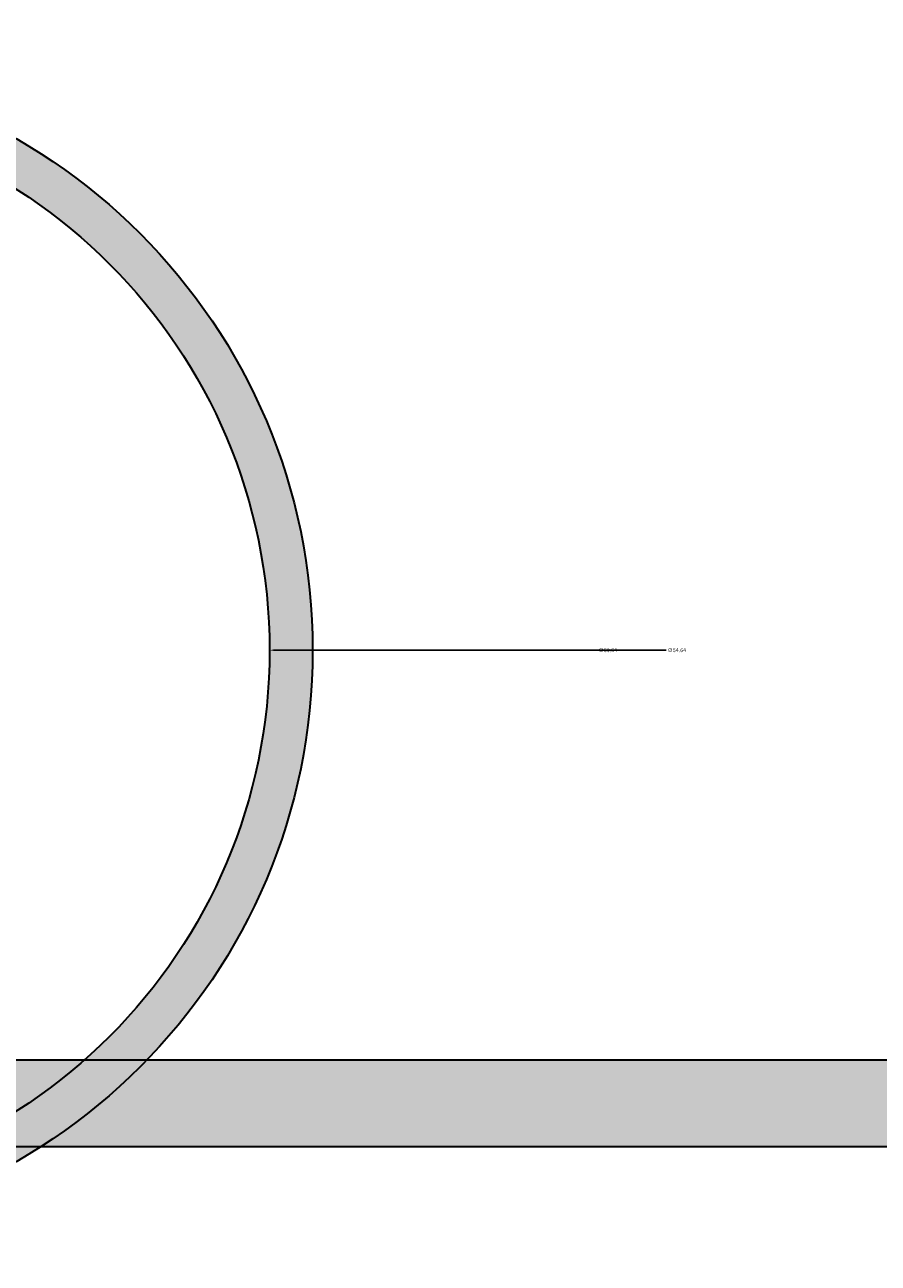
# Model space of a CAD drawing. Units: millimetres. Extents: x 446512 to 447461, y 70395 to 70610.
# Tile 31 of 39: x 447300 to 447340, y 70447 to 70505. Entities that reach past the tile are written whole.
import ezdxf

# ---------------------------------------------------------------- set-up
doc = ezdxf.new("R2010")
doc.units = ezdxf.units.MM
for name, color, linetype, lineweight in [('A-ANNO-DIMS', 2, 'Continuous', 18), ('A-FURN', 7, 'Continuous', 35), ('A-FURN-PATT', 38, 'Continuous', 13)]:
    doc.layers.add(name, color=color, linetype=linetype, lineweight=lineweight)
doc.styles.get("Standard").update_dxf_attribs({"font": 'arial.ttf'})
doc.dimstyles.get("Standard").update_dxf_attribs({"dimtxt": 0.18, "dimasz": 0.18, "dimexe": 0.18, "dimexo": 0.0625, "dimgap": 0.09, "dimtad": 0, "dimtih": 1, "dimtoh": 1, "dimdec": 4, "dimzin": 0, "dimdsep": 46, "dimtxsty": 'Standard', "dimcen": 0.09, "dimadec": 0, "dimazin": 0, "dimtfac": 1, "dimtdec": 4, "dimtofl": 0, "dimtmove": 0, "dimatfit": 3, "dimfxl": 1, "dimtolj": 1, "dimtzin": 0, "dimarcsym": 0})

# ---------------------------------------------------------------- blocks, each defined once
blk = doc.blocks.new('*D61')
at = {"layer": 'A-ANNO-DIMS', "color": 0, "lineweight": -2, "transparency": 16777216}
for p, q in [((447254.943, 70452.792), (447254.943, 70394.885)), ((447450.532, 70432.19), (447450.532, 70394.885)), ((447255.123, 70395.065), (447352.352, 70395.065)), ((447450.352, 70395.065), (447353.122, 70395.065))]:
    blk.add_line(p, q, dxfattribs=at)
at = {"layer": 'A-ANNO-DIMS', "color": 0, "transparency": 16777216}
for points in [[(447255.123, 70395.095), (447255.123, 70395.035), (447254.943, 70395.065)], [(447450.352, 70395.095), (447450.352, 70395.035), (447450.532, 70395.065)]]:
    blk.add_solid(points, dxfattribs=at)
at = {"layer": 'Defpoints', "color": 0, "transparency": 16777216}
for p in [(447254.943, 70452.855), (447450.532, 70432.253), (447450.532, 70395.065)]:
    blk.add_point(p, dxfattribs=at)
at = {"layer": 'A-ANNO-DIMS', "color": 0, "transparency": 16777216, "insert": (447352.737, 70395.065), "char_height": 0.18, "attachment_point": 5}
blk.add_mtext('\\A1;195.6', dxfattribs=at)
blk = doc.blocks.new('*D63')
at = {"layer": 'A-ANNO-DIMS', "color": 0, "lineweight": -2, "transparency": 16777216}
for p, q in [((447286.509, 70475.943), (447286.509, 70610.145)), ((447340.049, 70506.612), (447340.049, 70610.145)), ((447286.689, 70609.965), (447312.886, 70609.965)), ((447339.869, 70609.965), (447313.672, 70609.965))]:
    blk.add_line(p, q, dxfattribs=at)
at = {"layer": 'A-ANNO-DIMS', "color": 0, "transparency": 16777216}
for points in [[(447286.689, 70609.995), (447286.689, 70609.935), (447286.509, 70609.965)], [(447339.869, 70609.995), (447339.869, 70609.935), (447340.049, 70609.965)]]:
    blk.add_solid(points, dxfattribs=at)
at = {"layer": 'Defpoints', "color": 0, "transparency": 16777216}
for p in [(447340.049, 70609.965), (447340.049, 70506.55), (447286.509, 70475.881)]:
    blk.add_point(p, dxfattribs=at)
at = {"layer": 'A-ANNO-DIMS', "color": 0, "transparency": 16777216, "insert": (447313.279, 70609.965), "char_height": 0.18, "attachment_point": 5}
blk.add_mtext('\\A1;53.54', dxfattribs=at)
blk = doc.blocks.new('*D72')
at = {"layer": 'A-ANNO-DIMS', "color": 0, "lineweight": -2, "transparency": 16777216}
for p, q in [((447254.88, 70452.855), (447244.513, 70452.855)), ((447244.693, 70452.675), (447244.693, 70429.266)), ((447244.693, 70405.495), (447244.693, 70428.903)), ((447365.363, 70405.315), (447244.513, 70405.315))]:
    blk.add_line(p, q, dxfattribs=at)
at = {"layer": 'A-ANNO-DIMS', "color": 0, "transparency": 16777216}
for points in [[(447244.663, 70452.675), (447244.723, 70452.675), (447244.693, 70452.855)], [(447244.663, 70405.495), (447244.723, 70405.495), (447244.693, 70405.315)]]:
    blk.add_solid(points, dxfattribs=at)
at = {"layer": 'Defpoints', "color": 0, "transparency": 16777216}
for p in [(447244.693, 70452.855), (447254.943, 70452.855), (447365.425, 70405.315)]:
    blk.add_point(p, dxfattribs=at)
at = {"layer": 'A-ANNO-DIMS', "color": 0, "transparency": 16777216, "insert": (447244.693, 70429.085), "char_height": 0.18, "attachment_point": 5}
blk.add_mtext('\\A1;47.54', dxfattribs=at)
blk = doc.blocks.new('*D79')
at = {"layer": 'A-ANNO-DIMS', "color": 0, "lineweight": -2, "transparency": 16777216}
for p, q in [((447286.419, 70475.881), (447286.599, 70475.881)), ((447286.509, 70475.791), (447286.509, 70475.971)), ((447330.218, 70475.881), (447314.007, 70475.881))]:
    blk.add_line(p, q, dxfattribs=at)
at = {"layer": 'A-ANNO-DIMS', "color": 0, "transparency": 16777216}
blk.add_solid([(447314.007, 70475.911), (447314.007, 70475.851), (447313.827, 70475.881)], dxfattribs=at)
at = {"layer": 'Defpoints', "color": 0, "transparency": 16777216}
for p in [(447259.19, 70475.88), (447313.827, 70475.881)]:
    blk.add_point(p, dxfattribs=at)
at = {"layer": 'A-ANNO-DIMS', "color": 0, "transparency": 16777216, "insert": (447330.709, 70475.881), "char_height": 0.18, "attachment_point": 5}
blk.add_mtext('\\A1;∅54.64', dxfattribs=at)
blk = doc.blocks.new('*D80')
at = {"layer": 'A-ANNO-DIMS', "color": 0, "lineweight": -2, "transparency": 16777216}
for p, q in [((447286.419, 70475.881), (447286.599, 70475.881)), ((447286.509, 70475.791), (447286.509, 70475.971)), ((447327.018, 70475.881), (447312.007, 70475.881))]:
    blk.add_line(p, q, dxfattribs=at)
at = {"layer": 'A-ANNO-DIMS', "color": 0, "transparency": 16777216}
blk.add_solid([(447312.007, 70475.911), (447312.007, 70475.851), (447311.827, 70475.881)], dxfattribs=at)
at = {"layer": 'Defpoints', "color": 0, "transparency": 16777216}
for p in [(447261.19, 70475.88), (447311.827, 70475.881)]:
    blk.add_point(p, dxfattribs=at)
at = {"layer": 'A-ANNO-DIMS', "color": 0, "transparency": 16777216, "insert": (447327.509, 70475.881), "char_height": 0.18, "attachment_point": 5}
blk.add_mtext('\\A1;∅50.64', dxfattribs=at)

msp = doc.modelspace()

# ---------------------------------------------------------------- hatches: boundary and pattern name
at = {"layer": 'A-FURN-PATT'}
h = msp.add_hatch(color=256, dxfattribs=at)
h.dxf.hatch_style = 1
h.paths.add_polyline_path([(447259.1901, 70475.8806, 0.1945594), (447266.8704, 70456.89), (447269.7639, 70456.89, -0.2152771), (447261.1901, 70475.8806, -1), (447311.827, 70475.8806, -0.2152771), (447303.2532, 70456.89), (447306.1467, 70456.89, 0.1945594), (447313.827, 70475.8806, 1)])
h.paths.add_polyline_path([(447301.2097, 70452.855), (447297.037, 70452.855, -0.2177821), (447275.9801, 70452.855), (447271.8074, 70452.855, 0.2920128)])
h.paths.add_polyline_path([(447269.7639, 70456.89), (447266.8704, 70456.89, 0.0585505), (447271.8074, 70452.855), (447275.9801, 70452.855, -0.0735735)])
h.paths.add_polyline_path([(447306.1467, 70456.89), (447303.2532, 70456.89, -0.0735735), (447297.037, 70452.855), (447301.2097, 70452.855, 0.0585505)])
h = msp.add_hatch(color=256, dxfattribs=at)
h.dxf.hatch_style = 1
h.paths.add_polyline_path([(447280.3184, 70456.89), (447254.9427, 70456.89), (447254.9427, 70452.855), (447280.3184, 70452.855)])
h.paths.add_polyline_path([(447365.4251, 70456.89), (447340.9075, 70456.89), (447340.9075, 70452.855), (447365.4251, 70452.855)])
h.paths.add_polyline_path([(447340.9075, 70456.89), (447280.3184, 70456.89), (447280.3184, 70452.855), (447340.9075, 70452.855)])

# ---------------------------------------------------------------- linework, layer by layer
at = {"layer": 'A-FURN'}
msp.add_lwpolyline([(447254.9427, 70456.89), (447365.4251, 70456.89), (447365.4251, 70452.855), (447254.9427, 70452.855)], close=True, dxfattribs=at)
for radius in [27.3185, 25.3185]:
    msp.add_circle((447286.5086, 70475.8806), radius, dxfattribs=at)

# ---------------------------------------------------------------- dimensions: what is measured, and where the dimension line sits
at = {"layer": 'A-ANNO-DIMS'}
for base, p1, p2, override, picture, middle in [((447340.0494, 70609.9647), (447286.5086, 70475.8806), (447340.0494, 70506.5496), {"dimdec": 2, "dimlfac": 1, "dimrnd": 0, "dimzin": 0, "dimdsep": 46, "dimlunit": 2}, '*D63', (447313.279, 70609.9647)), ((447450.5318, 70395.0645), (447254.9427, 70452.855), (447450.5318, 70432.2526), {"dimdec": 1, "dimlfac": 1, "dimrnd": 0, "dimzin": 0, "dimdsep": 46, "dimlunit": 2}, '*D61', (447352.7372, 70395.0645))]:
    dim = msp.add_linear_dim(base=base, p1=p1, p2=p2, dimstyle='Standard', override=override, dxfattribs=at)
    dim.commit()
    dim.dimension.update_dxf_attribs({"geometry": picture, "text_midpoint": middle})
for p1, p2, picture, middle in [((447259.1901, 70475.8801), (447313.827, 70475.881), '*D79', (447330.2181, 70475.8813)), ((447261.1901, 70475.8801), (447311.827, 70475.881), '*D80', (447327.0181, 70475.8813))]:
    dim = msp.add_diameter_dim_2p(p1=p1, p2=p2, dimstyle='Standard', override={"dimdec": 2, "dimlfac": 1, "dimrnd": 0, "dimzin": 0, "dimdsep": 46, "dimlunit": 2}, dxfattribs=at)
    dim.commit()
    dim.dimension.update_dxf_attribs({"geometry": picture, "text_midpoint": middle, "dimtype": 163})
dim = msp.add_linear_dim(base=(447244.6927, 70452.855), p1=(447365.4251, 70405.3145), p2=(447254.9427, 70452.855), angle=90, dimstyle='Standard', override={"dimdec": 2, "dimlfac": 1, "dimrnd": 0, "dimzin": 0, "dimdsep": 46, "dimlunit": 2}, dxfattribs=at)
dim.commit()
dim.dimension.update_dxf_attribs({"geometry": '*D72', "text_midpoint": (447244.6927, 70429.0848)})

doc.saveas('drawing.dxf')
